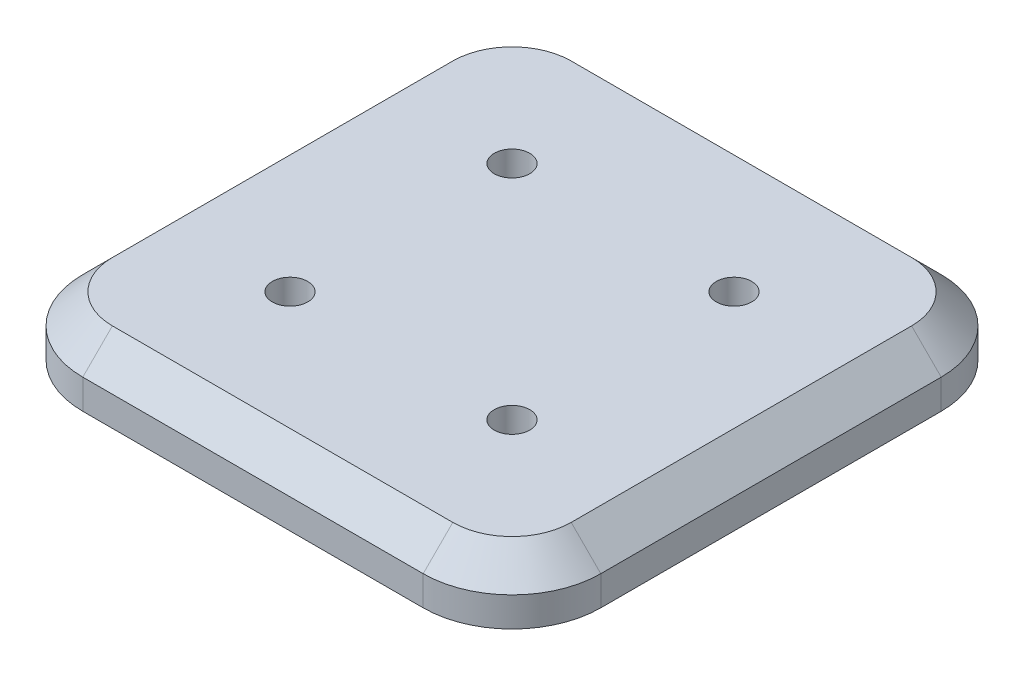
ISO-10303-21;
HEADER;
FILE_DESCRIPTION(('STEP AP214'),'2;1');
FILE_NAME('part.step','',(''),(''),'','','');
FILE_SCHEMA(('AUTOMOTIVE_DESIGN { 1 0 10303 214 1 1 1 1 }'));
ENDSEC;
DATA;
#1=APPLICATION_CONTEXT('core data for automotive mechanical design processes');
#2=APPLICATION_PROTOCOL_DEFINITION('international standard','automotive_design',2000,#1);
#3=PRODUCT_CONTEXT('',#1,'mechanical');
#4=PRODUCT('Part','Part','',(#3));
#5=PRODUCT_RELATED_PRODUCT_CATEGORY('part','',(#4));
#6=PRODUCT_DEFINITION_FORMATION('','',#4);
#7=PRODUCT_DEFINITION_CONTEXT('part definition',#1,'design');
#8=PRODUCT_DEFINITION('design','',#6,#7);
#9=PRODUCT_DEFINITION_SHAPE('','',#8);
#10=(LENGTH_UNIT() NAMED_UNIT(*) SI_UNIT(.MILLI.,.METRE.));
#11=(NAMED_UNIT(*) PLANE_ANGLE_UNIT() SI_UNIT($,.RADIAN.));
#12=(NAMED_UNIT(*) SI_UNIT($,.STERADIAN.) SOLID_ANGLE_UNIT());
#13=UNCERTAINTY_MEASURE_WITH_UNIT(LENGTH_MEASURE(1.E-05),#10,'distance_accuracy_value','');
#14=(GEOMETRIC_REPRESENTATION_CONTEXT(3) GLOBAL_UNCERTAINTY_ASSIGNED_CONTEXT((#13)) GLOBAL_UNIT_ASSIGNED_CONTEXT((#10,
#11,#12)) REPRESENTATION_CONTEXT('',''));
#15=CARTESIAN_POINT('',(0.,0.,0.));
#16=DIRECTION('',(0.,0.,1.));
#17=DIRECTION('',(1.,0.,0.));
#18=AXIS2_PLACEMENT_3D('',#15,#16,#17);
#19=CARTESIAN_POINT('',(87.5,20.,87.5));
#20=DIRECTION('',(-1.,0.,0.));
#21=DIRECTION('',(0.,0.,1.));
#22=AXIS2_PLACEMENT_3D('',#19,#20,#21);
#23=PLANE('',#22);
#24=DIRECTION('',(0.,-1.,0.));
#25=VECTOR('',#24,1.);
#26=CARTESIAN_POINT('',(87.5,20.,-57.5));
#27=LINE('',#26,#25);
#28=CARTESIAN_POINT('',(87.5,0.,-57.5));
#29=VERTEX_POINT('',#28);
#30=CARTESIAN_POINT('',(87.5,9.99999999999994,-57.5));
#31=VERTEX_POINT('',#30);
#32=EDGE_CURVE('E242',#29,#31,#27,.F.);
#33=ORIENTED_EDGE('',*,*,#32,.T.);
#34=DIRECTION('',(0.,0.,1.));
#35=VECTOR('',#34,1.);
#36=CARTESIAN_POINT('',(87.5,9.99999999999994,87.5));
#37=LINE('',#36,#35);
#38=CARTESIAN_POINT('',(87.5,9.99999999999994,57.5));
#39=VERTEX_POINT('',#38);
#40=EDGE_CURVE('E280',#31,#39,#37,.T.);
#41=ORIENTED_EDGE('',*,*,#40,.T.);
#42=DIRECTION('',(0.,-1.,0.));
#43=VECTOR('',#42,1.);
#44=CARTESIAN_POINT('',(87.5,20.,57.5));
#45=LINE('',#44,#43);
#46=CARTESIAN_POINT('',(87.5,0.,57.5));
#47=VERTEX_POINT('',#46);
#48=EDGE_CURVE('E245',#39,#47,#45,.T.);
#49=ORIENTED_EDGE('',*,*,#48,.T.);
#50=DIRECTION('',(0.,0.,-1.));
#51=VECTOR('',#50,1.);
#52=CARTESIAN_POINT('',(87.5,0.,87.5));
#53=LINE('',#52,#51);
#54=EDGE_CURVE('E215',#47,#29,#53,.T.);
#55=ORIENTED_EDGE('',*,*,#54,.T.);
#56=EDGE_LOOP('',(#33,#41,#49,#55));
#57=FACE_BOUND('',#56,.T.);
#58=ADVANCED_FACE('F41',(#57),#23,.F.);
#59=CARTESIAN_POINT('',(-87.5,20.,-87.5));
#60=DIRECTION('',(0.,0.,1.));
#61=DIRECTION('',(1.,0.,0.));
#62=AXIS2_PLACEMENT_3D('',#59,#60,#61);
#63=PLANE('',#62);
#64=DIRECTION('',(0.,-1.,0.));
#65=VECTOR('',#64,1.);
#66=CARTESIAN_POINT('',(-57.5,20.,-87.5));
#67=LINE('',#66,#65);
#68=CARTESIAN_POINT('',(-57.5,0.,-87.5));
#69=VERTEX_POINT('',#68);
#70=CARTESIAN_POINT('',(-57.5,9.99999999999994,-87.5));
#71=VERTEX_POINT('',#70);
#72=EDGE_CURVE('E237',#69,#71,#67,.F.);
#73=ORIENTED_EDGE('',*,*,#72,.T.);
#74=DIRECTION('',(1.,0.,0.));
#75=VECTOR('',#74,1.);
#76=CARTESIAN_POINT('',(-87.5,9.99999999999994,-87.5));
#77=LINE('',#76,#75);
#78=CARTESIAN_POINT('',(57.5,9.99999999999994,-87.5));
#79=VERTEX_POINT('',#78);
#80=EDGE_CURVE('E268',#71,#79,#77,.T.);
#81=ORIENTED_EDGE('',*,*,#80,.T.);
#82=DIRECTION('',(0.,-1.,0.));
#83=VECTOR('',#82,1.);
#84=CARTESIAN_POINT('',(57.5,20.,-87.5));
#85=LINE('',#84,#83);
#86=CARTESIAN_POINT('',(57.5,0.,-87.5));
#87=VERTEX_POINT('',#86);
#88=EDGE_CURVE('E240',#79,#87,#85,.T.);
#89=ORIENTED_EDGE('',*,*,#88,.T.);
#90=DIRECTION('',(-1.,0.,0.));
#91=VECTOR('',#90,1.);
#92=CARTESIAN_POINT('',(-87.5,0.,-87.5));
#93=LINE('',#92,#91);
#94=EDGE_CURVE('E213',#87,#69,#93,.T.);
#95=ORIENTED_EDGE('',*,*,#94,.T.);
#96=EDGE_LOOP('',(#73,#81,#89,#95));
#97=FACE_BOUND('',#96,.T.);
#98=ADVANCED_FACE('F346',(#97),#63,.F.);
#99=CARTESIAN_POINT('',(-87.5,20.,87.5));
#100=DIRECTION('',(1.,0.,0.));
#101=DIRECTION('',(0.,0.,-1.));
#102=AXIS2_PLACEMENT_3D('',#99,#100,#101);
#103=PLANE('',#102);
#104=DIRECTION('',(0.,-1.,0.));
#105=VECTOR('',#104,1.);
#106=CARTESIAN_POINT('',(-87.5,20.,57.5));
#107=LINE('',#106,#105);
#108=CARTESIAN_POINT('',(-87.5,0.,57.5));
#109=VERTEX_POINT('',#108);
#110=CARTESIAN_POINT('',(-87.5,9.99999999999994,57.5));
#111=VERTEX_POINT('',#110);
#112=EDGE_CURVE('E222',#109,#111,#107,.F.);
#113=ORIENTED_EDGE('',*,*,#112,.T.);
#114=DIRECTION('',(0.,0.,-1.));
#115=VECTOR('',#114,1.);
#116=CARTESIAN_POINT('',(-87.5,9.99999999999994,87.5));
#117=LINE('',#116,#115);
#118=CARTESIAN_POINT('',(-87.5,9.99999999999994,-57.5));
#119=VERTEX_POINT('',#118);
#120=EDGE_CURVE('E273',#111,#119,#117,.T.);
#121=ORIENTED_EDGE('',*,*,#120,.T.);
#122=DIRECTION('',(0.,-1.,0.));
#123=VECTOR('',#122,1.);
#124=CARTESIAN_POINT('',(-87.5,20.,-57.5));
#125=LINE('',#124,#123);
#126=CARTESIAN_POINT('',(-87.5,0.,-57.5));
#127=VERTEX_POINT('',#126);
#128=EDGE_CURVE('E227',#119,#127,#125,.T.);
#129=ORIENTED_EDGE('',*,*,#128,.T.);
#130=DIRECTION('',(0.,0.,1.));
#131=VECTOR('',#130,1.);
#132=CARTESIAN_POINT('',(-87.5,0.,87.5));
#133=LINE('',#132,#131);
#134=EDGE_CURVE('E218',#127,#109,#133,.T.);
#135=ORIENTED_EDGE('',*,*,#134,.T.);
#136=EDGE_LOOP('',(#113,#121,#129,#135));
#137=FACE_BOUND('',#136,.T.);
#138=ADVANCED_FACE('F319',(#137),#103,.F.);
#139=CARTESIAN_POINT('',(-87.5,20.,87.5));
#140=DIRECTION('',(0.,0.,-1.));
#141=DIRECTION('',(-1.,0.,0.));
#142=AXIS2_PLACEMENT_3D('',#139,#140,#141);
#143=PLANE('',#142);
#144=DIRECTION('',(0.,-1.,0.));
#145=VECTOR('',#144,1.);
#146=CARTESIAN_POINT('',(57.5,20.,87.5));
#147=LINE('',#146,#145);
#148=CARTESIAN_POINT('',(57.5,0.,87.5));
#149=VERTEX_POINT('',#148);
#150=CARTESIAN_POINT('',(57.5,9.99999999999994,87.5));
#151=VERTEX_POINT('',#150);
#152=EDGE_CURVE('E248',#149,#151,#147,.F.);
#153=ORIENTED_EDGE('',*,*,#152,.T.);
#154=DIRECTION('',(-1.,0.,0.));
#155=VECTOR('',#154,1.);
#156=CARTESIAN_POINT('',(-87.5,9.99999999999994,87.5));
#157=LINE('',#156,#155);
#158=CARTESIAN_POINT('',(-57.5,9.99999999999994,87.5));
#159=VERTEX_POINT('',#158);
#160=EDGE_CURVE('E11',#151,#159,#157,.T.);
#161=ORIENTED_EDGE('',*,*,#160,.T.);
#162=DIRECTION('',(0.,-1.,0.));
#163=VECTOR('',#162,1.);
#164=CARTESIAN_POINT('',(-57.5,20.,87.5));
#165=LINE('',#164,#163);
#166=CARTESIAN_POINT('',(-57.5,0.,87.5));
#167=VERTEX_POINT('',#166);
#168=EDGE_CURVE('E250',#159,#167,#165,.T.);
#169=ORIENTED_EDGE('',*,*,#168,.T.);
#170=DIRECTION('',(1.,0.,0.));
#171=VECTOR('',#170,1.);
#172=CARTESIAN_POINT('',(-87.5,0.,87.5));
#173=LINE('',#172,#171);
#174=EDGE_CURVE('E221',#167,#149,#173,.T.);
#175=ORIENTED_EDGE('',*,*,#174,.T.);
#176=EDGE_LOOP('',(#153,#161,#169,#175));
#177=FACE_BOUND('',#176,.T.);
#178=ADVANCED_FACE('F328',(#177),#143,.F.);
#179=CARTESIAN_POINT('',(0.,20.,0.));
#180=DIRECTION('',(0.,-1.,0.));
#181=DIRECTION('',(0.,0.,-1.));
#182=AXIS2_PLACEMENT_3D('',#179,#180,#181);
#183=PLANE('',#182);
#184=CARTESIAN_POINT('',(-37.5,20.,-37.5));
#185=DIRECTION('',(0.,1.,0.));
#186=DIRECTION('',(0.,0.,1.));
#187=AXIS2_PLACEMENT_3D('',#184,#185,#186);
#188=CIRCLE('',#187,5.99999999999998);
#189=CARTESIAN_POINT('',(-37.5,20.,-31.5));
#190=VERTEX_POINT('',#189);
#191=EDGE_CURVE('E190',#190,#190,#188,.T.);
#192=ORIENTED_EDGE('',*,*,#191,.F.);
#193=EDGE_LOOP('',(#192));
#194=FACE_BOUND('',#193,.T.);
#195=CARTESIAN_POINT('',(37.5,20.,-37.5));
#196=DIRECTION('',(0.,1.,0.));
#197=DIRECTION('',(0.,0.,1.));
#198=AXIS2_PLACEMENT_3D('',#195,#196,#197);
#199=CIRCLE('',#198,5.99999999999998);
#200=CARTESIAN_POINT('',(37.5,20.,-31.5));
#201=VERTEX_POINT('',#200);
#202=EDGE_CURVE('E194',#201,#201,#199,.T.);
#203=ORIENTED_EDGE('',*,*,#202,.F.);
#204=EDGE_LOOP('',(#203));
#205=FACE_BOUND('',#204,.T.);
#206=CARTESIAN_POINT('',(37.5,20.,37.5));
#207=DIRECTION('',(0.,1.,0.));
#208=DIRECTION('',(0.,0.,1.));
#209=AXIS2_PLACEMENT_3D('',#206,#207,#208);
#210=CIRCLE('',#209,5.99999999999998);
#211=CARTESIAN_POINT('',(37.5,20.,43.5));
#212=VERTEX_POINT('',#211);
#213=EDGE_CURVE('E197',#212,#212,#210,.T.);
#214=ORIENTED_EDGE('',*,*,#213,.F.);
#215=EDGE_LOOP('',(#214));
#216=FACE_BOUND('',#215,.T.);
#217=CARTESIAN_POINT('',(-37.5,20.,37.5));
#218=DIRECTION('',(0.,1.,0.));
#219=DIRECTION('',(0.,0.,1.));
#220=AXIS2_PLACEMENT_3D('',#217,#218,#219);
#221=CIRCLE('',#220,5.99999999999998);
#222=CARTESIAN_POINT('',(-37.5,20.,43.5));
#223=VERTEX_POINT('',#222);
#224=EDGE_CURVE('E204',#223,#223,#221,.T.);
#225=ORIENTED_EDGE('',*,*,#224,.F.);
#226=EDGE_LOOP('',(#225));
#227=FACE_BOUND('',#226,.T.);
#228=CARTESIAN_POINT('',(57.5,20.,-57.5));
#229=DIRECTION('',(0.,-1.,0.));
#230=DIRECTION('',(0.,0.,-1.));
#231=AXIS2_PLACEMENT_3D('',#228,#229,#230);
#232=CIRCLE('',#231,20.);
#233=CARTESIAN_POINT('',(77.5,20.,-57.5));
#234=VERTEX_POINT('',#233);
#235=CARTESIAN_POINT('',(57.5,20.,-77.5));
#236=VERTEX_POINT('',#235);
#237=EDGE_CURVE('E261',#234,#236,#232,.F.);
#238=ORIENTED_EDGE('',*,*,#237,.T.);
#239=DIRECTION('',(-1.,0.,0.));
#240=VECTOR('',#239,1.);
#241=CARTESIAN_POINT('',(0.,20.,-77.5));
#242=LINE('',#241,#240);
#243=CARTESIAN_POINT('',(-57.5,20.,-77.5));
#244=VERTEX_POINT('',#243);
#245=EDGE_CURVE('E264',#236,#244,#242,.T.);
#246=ORIENTED_EDGE('',*,*,#245,.T.);
#247=CARTESIAN_POINT('',(-57.5,20.,-57.5));
#248=DIRECTION('',(0.,-1.,0.));
#249=DIRECTION('',(0.,0.,-1.));
#250=AXIS2_PLACEMENT_3D('',#247,#248,#249);
#251=CIRCLE('',#250,20.);
#252=CARTESIAN_POINT('',(-77.5,20.,-57.5));
#253=VERTEX_POINT('',#252);
#254=EDGE_CURVE('E263',#244,#253,#251,.F.);
#255=ORIENTED_EDGE('',*,*,#254,.T.);
#256=DIRECTION('',(0.,0.,1.));
#257=VECTOR('',#256,1.);
#258=CARTESIAN_POINT('',(-77.5,20.,0.));
#259=LINE('',#258,#257);
#260=CARTESIAN_POINT('',(-77.5,20.,57.5));
#261=VERTEX_POINT('',#260);
#262=EDGE_CURVE('E256',#253,#261,#259,.T.);
#263=ORIENTED_EDGE('',*,*,#262,.T.);
#264=CARTESIAN_POINT('',(-57.5,20.,57.5));
#265=DIRECTION('',(0.,-1.,0.));
#266=DIRECTION('',(0.,0.,-1.));
#267=AXIS2_PLACEMENT_3D('',#264,#265,#266);
#268=CIRCLE('',#267,20.);
#269=CARTESIAN_POINT('',(-57.5,20.,77.5));
#270=VERTEX_POINT('',#269);
#271=EDGE_CURVE('E253',#261,#270,#268,.F.);
#272=ORIENTED_EDGE('',*,*,#271,.T.);
#273=DIRECTION('',(1.,0.,0.));
#274=VECTOR('',#273,1.);
#275=CARTESIAN_POINT('',(0.,20.,77.5));
#276=LINE('',#275,#274);
#277=CARTESIAN_POINT('',(57.5,20.,77.5));
#278=VERTEX_POINT('',#277);
#279=EDGE_CURVE('E252',#270,#278,#276,.T.);
#280=ORIENTED_EDGE('',*,*,#279,.T.);
#281=CARTESIAN_POINT('',(57.5,20.,57.5));
#282=DIRECTION('',(0.,-1.,0.));
#283=DIRECTION('',(0.,0.,-1.));
#284=AXIS2_PLACEMENT_3D('',#281,#282,#283);
#285=CIRCLE('',#284,20.);
#286=CARTESIAN_POINT('',(77.5,20.,57.5));
#287=VERTEX_POINT('',#286);
#288=EDGE_CURVE('E254',#278,#287,#285,.F.);
#289=ORIENTED_EDGE('',*,*,#288,.T.);
#290=DIRECTION('',(0.,0.,-1.));
#291=VECTOR('',#290,1.);
#292=CARTESIAN_POINT('',(77.5,20.,0.));
#293=LINE('',#292,#291);
#294=EDGE_CURVE('E260',#287,#234,#293,.T.);
#295=ORIENTED_EDGE('',*,*,#294,.T.);
#296=EDGE_LOOP('',(#238,#246,#255,#263,#272,#280,#289,#295));
#297=FACE_BOUND('',#296,.T.);
#298=ADVANCED_FACE('F356',(#194,#205,#216,#227,#297),#183,.F.);
#299=CARTESIAN_POINT('',(0.,0.,0.));
#300=DIRECTION('',(0.,-1.,0.));
#301=DIRECTION('',(0.,0.,-1.));
#302=AXIS2_PLACEMENT_3D('',#299,#300,#301);
#303=PLANE('',#302);
#304=CARTESIAN_POINT('',(-62.5,0.,62.5));
#305=DIRECTION('',(0.,-1.,0.));
#306=DIRECTION('',(0.,0.,-1.));
#307=AXIS2_PLACEMENT_3D('',#304,#305,#306);
#308=CIRCLE('',#307,5.99999999999998);
#309=CARTESIAN_POINT('',(-62.5,0.,56.5));
#310=VERTEX_POINT('',#309);
#311=EDGE_CURVE('E164',#310,#310,#308,.T.);
#312=ORIENTED_EDGE('',*,*,#311,.F.);
#313=EDGE_LOOP('',(#312));
#314=FACE_BOUND('',#313,.T.);
#315=CARTESIAN_POINT('',(62.5,0.,62.5));
#316=DIRECTION('',(0.,-1.,0.));
#317=DIRECTION('',(0.,0.,-1.));
#318=AXIS2_PLACEMENT_3D('',#315,#316,#317);
#319=CIRCLE('',#318,5.99999999999999);
#320=CARTESIAN_POINT('',(62.5,0.,56.5));
#321=VERTEX_POINT('',#320);
#322=EDGE_CURVE('E165',#321,#321,#319,.T.);
#323=ORIENTED_EDGE('',*,*,#322,.F.);
#324=EDGE_LOOP('',(#323));
#325=FACE_BOUND('',#324,.T.);
#326=CARTESIAN_POINT('',(62.5,0.,-62.5));
#327=DIRECTION('',(0.,-1.,0.));
#328=DIRECTION('',(0.,0.,-1.));
#329=AXIS2_PLACEMENT_3D('',#326,#327,#328);
#330=CIRCLE('',#329,5.99999999999999);
#331=CARTESIAN_POINT('',(62.5,0.,-68.5));
#332=VERTEX_POINT('',#331);
#333=EDGE_CURVE('E174',#332,#332,#330,.T.);
#334=ORIENTED_EDGE('',*,*,#333,.F.);
#335=EDGE_LOOP('',(#334));
#336=FACE_BOUND('',#335,.T.);
#337=CARTESIAN_POINT('',(-62.5,0.,-62.5));
#338=DIRECTION('',(0.,-1.,0.));
#339=DIRECTION('',(0.,0.,-1.));
#340=AXIS2_PLACEMENT_3D('',#337,#338,#339);
#341=CIRCLE('',#340,5.99999999999998);
#342=CARTESIAN_POINT('',(-62.5,0.,-68.5));
#343=VERTEX_POINT('',#342);
#344=EDGE_CURVE('E181',#343,#343,#341,.T.);
#345=ORIENTED_EDGE('',*,*,#344,.F.);
#346=EDGE_LOOP('',(#345));
#347=FACE_BOUND('',#346,.T.);
#348=ORIENTED_EDGE('',*,*,#134,.F.);
#349=CARTESIAN_POINT('',(-57.5,0.,-57.5));
#350=DIRECTION('',(0.,-1.,0.));
#351=DIRECTION('',(0.,0.,-1.));
#352=AXIS2_PLACEMENT_3D('',#349,#350,#351);
#353=CIRCLE('',#352,30.);
#354=EDGE_CURVE('E232',#127,#69,#353,.T.);
#355=ORIENTED_EDGE('',*,*,#354,.T.);
#356=ORIENTED_EDGE('',*,*,#94,.F.);
#357=CARTESIAN_POINT('',(57.5,0.,-57.5));
#358=DIRECTION('',(0.,-1.,0.));
#359=DIRECTION('',(0.,0.,-1.));
#360=AXIS2_PLACEMENT_3D('',#357,#358,#359);
#361=CIRCLE('',#360,30.);
#362=EDGE_CURVE('E231',#87,#29,#361,.T.);
#363=ORIENTED_EDGE('',*,*,#362,.T.);
#364=ORIENTED_EDGE('',*,*,#54,.F.);
#365=CARTESIAN_POINT('',(57.5,0.,57.5));
#366=DIRECTION('',(0.,-1.,0.));
#367=DIRECTION('',(0.,0.,-1.));
#368=AXIS2_PLACEMENT_3D('',#365,#366,#367);
#369=CIRCLE('',#368,30.);
#370=EDGE_CURVE('E233',#47,#149,#369,.T.);
#371=ORIENTED_EDGE('',*,*,#370,.T.);
#372=ORIENTED_EDGE('',*,*,#174,.F.);
#373=CARTESIAN_POINT('',(-57.5,0.,57.5));
#374=DIRECTION('',(0.,-1.,0.));
#375=DIRECTION('',(0.,0.,-1.));
#376=AXIS2_PLACEMENT_3D('',#373,#374,#375);
#377=CIRCLE('',#376,30.);
#378=EDGE_CURVE('E230',#167,#109,#377,.T.);
#379=ORIENTED_EDGE('',*,*,#378,.T.);
#380=EDGE_LOOP('',(#348,#355,#356,#363,#364,#371,#372,#379));
#381=FACE_BOUND('',#380,.T.);
#382=ADVANCED_FACE('F324',(#314,#325,#336,#347,#381),#303,.T.);
#383=CARTESIAN_POINT('',(-57.5,20.,-57.5));
#384=DIRECTION('',(0.,-1.,0.));
#385=DIRECTION('',(0.,0.,-1.));
#386=AXIS2_PLACEMENT_3D('',#383,#384,#385);
#387=CYLINDRICAL_SURFACE('',#386,30.);
#388=ORIENTED_EDGE('',*,*,#128,.F.);
#389=CARTESIAN_POINT('',(-57.5,9.99999999999994,-57.5));
#390=DIRECTION('',(0.,-1.,0.));
#391=DIRECTION('',(0.,0.,-1.));
#392=AXIS2_PLACEMENT_3D('',#389,#390,#391);
#393=CIRCLE('',#392,30.);
#394=EDGE_CURVE('E272',#119,#71,#393,.T.);
#395=ORIENTED_EDGE('',*,*,#394,.T.);
#396=ORIENTED_EDGE('',*,*,#72,.F.);
#397=ORIENTED_EDGE('',*,*,#354,.F.);
#398=EDGE_LOOP('',(#388,#395,#396,#397));
#399=FACE_BOUND('',#398,.T.);
#400=ADVANCED_FACE('F382',(#399),#387,.T.);
#401=CARTESIAN_POINT('',(57.5,20.,-57.5));
#402=DIRECTION('',(0.,-1.,0.));
#403=DIRECTION('',(0.,0.,-1.));
#404=AXIS2_PLACEMENT_3D('',#401,#402,#403);
#405=CYLINDRICAL_SURFACE('',#404,30.);
#406=ORIENTED_EDGE('',*,*,#88,.F.);
#407=CARTESIAN_POINT('',(57.5,9.99999999999994,-57.5));
#408=DIRECTION('',(0.,-1.,0.));
#409=DIRECTION('',(0.,0.,-1.));
#410=AXIS2_PLACEMENT_3D('',#407,#408,#409);
#411=CIRCLE('',#410,30.);
#412=EDGE_CURVE('E271',#79,#31,#411,.T.);
#413=ORIENTED_EDGE('',*,*,#412,.T.);
#414=ORIENTED_EDGE('',*,*,#32,.F.);
#415=ORIENTED_EDGE('',*,*,#362,.F.);
#416=EDGE_LOOP('',(#406,#413,#414,#415));
#417=FACE_BOUND('',#416,.T.);
#418=ADVANCED_FACE('F337',(#417),#405,.T.);
#419=CARTESIAN_POINT('',(57.5,20.,57.5));
#420=DIRECTION('',(0.,-1.,0.));
#421=DIRECTION('',(0.,0.,-1.));
#422=AXIS2_PLACEMENT_3D('',#419,#420,#421);
#423=CYLINDRICAL_SURFACE('',#422,30.);
#424=ORIENTED_EDGE('',*,*,#48,.F.);
#425=CARTESIAN_POINT('',(57.5,9.99999999999994,57.5));
#426=DIRECTION('',(0.,-1.,0.));
#427=DIRECTION('',(0.,0.,-1.));
#428=AXIS2_PLACEMENT_3D('',#425,#426,#427);
#429=CIRCLE('',#428,30.);
#430=EDGE_CURVE('E51',#39,#151,#429,.T.);
#431=ORIENTED_EDGE('',*,*,#430,.T.);
#432=ORIENTED_EDGE('',*,*,#152,.F.);
#433=ORIENTED_EDGE('',*,*,#370,.F.);
#434=EDGE_LOOP('',(#424,#431,#432,#433));
#435=FACE_BOUND('',#434,.T.);
#436=ADVANCED_FACE('F327',(#435),#423,.T.);
#437=CARTESIAN_POINT('',(-57.5,20.,57.5));
#438=DIRECTION('',(0.,-1.,0.));
#439=DIRECTION('',(0.,0.,-1.));
#440=AXIS2_PLACEMENT_3D('',#437,#438,#439);
#441=CYLINDRICAL_SURFACE('',#440,30.);
#442=ORIENTED_EDGE('',*,*,#168,.F.);
#443=CARTESIAN_POINT('',(-57.5,9.99999999999994,57.5));
#444=DIRECTION('',(0.,-1.,0.));
#445=DIRECTION('',(0.,0.,-1.));
#446=AXIS2_PLACEMENT_3D('',#443,#444,#445);
#447=CIRCLE('',#446,30.);
#448=EDGE_CURVE('E276',#159,#111,#447,.T.);
#449=ORIENTED_EDGE('',*,*,#448,.T.);
#450=ORIENTED_EDGE('',*,*,#112,.F.);
#451=ORIENTED_EDGE('',*,*,#378,.F.);
#452=EDGE_LOOP('',(#442,#449,#450,#451));
#453=FACE_BOUND('',#452,.T.);
#454=ADVANCED_FACE('F314',(#453),#441,.T.);
#455=CARTESIAN_POINT('',(0.,20.,77.5));
#456=DIRECTION('',(0.,-0.707106781186545,-0.707106781186551));
#457=DIRECTION('',(1.,0.,0.));
#458=AXIS2_PLACEMENT_3D('',#455,#456,#457);
#459=PLANE('',#458);
#460=DIRECTION('',(0.,0.707106781186551,-0.707106781186545));
#461=VECTOR('',#460,1.);
#462=CARTESIAN_POINT('',(-57.5,9.99999999999994,87.5));
#463=LINE('',#462,#461);
#464=EDGE_CURVE('E298',#159,#270,#463,.T.);
#465=ORIENTED_EDGE('',*,*,#464,.F.);
#466=ORIENTED_EDGE('',*,*,#160,.F.);
#467=DIRECTION('',(0.,-0.707106781186551,0.707106781186545));
#468=VECTOR('',#467,1.);
#469=CARTESIAN_POINT('',(57.5,20.,77.5));
#470=LINE('',#469,#468);
#471=EDGE_CURVE('E46',#278,#151,#470,.T.);
#472=ORIENTED_EDGE('',*,*,#471,.F.);
#473=ORIENTED_EDGE('',*,*,#279,.F.);
#474=EDGE_LOOP('',(#465,#466,#472,#473));
#475=FACE_BOUND('',#474,.T.);
#476=ADVANCED_FACE('F42',(#475),#459,.F.);
#477=CARTESIAN_POINT('',(57.5,20.,57.5));
#478=DIRECTION('',(0.,-1.,0.));
#479=DIRECTION('',(0.,0.,-1.));
#480=AXIS2_PLACEMENT_3D('',#477,#478,#479);
#481=CONICAL_SURFACE('',#480,20.,0.785398163397444);
#482=ORIENTED_EDGE('',*,*,#471,.T.);
#483=ORIENTED_EDGE('',*,*,#430,.F.);
#484=DIRECTION('',(0.707106781186545,-0.707106781186551,0.));
#485=VECTOR('',#484,1.);
#486=CARTESIAN_POINT('',(77.5,20.,57.5));
#487=LINE('',#486,#485);
#488=EDGE_CURVE('E295',#287,#39,#487,.T.);
#489=ORIENTED_EDGE('',*,*,#488,.F.);
#490=ORIENTED_EDGE('',*,*,#288,.F.);
#491=EDGE_LOOP('',(#482,#483,#489,#490));
#492=FACE_BOUND('',#491,.T.);
#493=ADVANCED_FACE('F306',(#492),#481,.T.);
#494=CARTESIAN_POINT('',(-57.5,20.,57.5));
#495=DIRECTION('',(0.,-1.,0.));
#496=DIRECTION('',(0.,0.,-1.));
#497=AXIS2_PLACEMENT_3D('',#494,#495,#496);
#498=CONICAL_SURFACE('',#497,20.,0.785398163397444);
#499=ORIENTED_EDGE('',*,*,#464,.T.);
#500=ORIENTED_EDGE('',*,*,#271,.F.);
#501=DIRECTION('',(0.707106781186545,0.707106781186551,0.));
#502=VECTOR('',#501,1.);
#503=CARTESIAN_POINT('',(-87.5,9.99999999999994,57.5));
#504=LINE('',#503,#502);
#505=EDGE_CURVE('E293',#111,#261,#504,.T.);
#506=ORIENTED_EDGE('',*,*,#505,.F.);
#507=ORIENTED_EDGE('',*,*,#448,.F.);
#508=EDGE_LOOP('',(#499,#500,#506,#507));
#509=FACE_BOUND('',#508,.T.);
#510=ADVANCED_FACE('F311',(#509),#498,.T.);
#511=CARTESIAN_POINT('',(77.5,20.,0.));
#512=DIRECTION('',(-0.707106781186551,-0.707106781186545,0.));
#513=DIRECTION('',(0.,0.,-1.));
#514=AXIS2_PLACEMENT_3D('',#511,#512,#513);
#515=PLANE('',#514);
#516=ORIENTED_EDGE('',*,*,#488,.T.);
#517=ORIENTED_EDGE('',*,*,#40,.F.);
#518=DIRECTION('',(0.707106781186545,-0.707106781186551,0.));
#519=VECTOR('',#518,1.);
#520=CARTESIAN_POINT('',(77.5,20.,-57.5));
#521=LINE('',#520,#519);
#522=EDGE_CURVE('E288',#234,#31,#521,.T.);
#523=ORIENTED_EDGE('',*,*,#522,.F.);
#524=ORIENTED_EDGE('',*,*,#294,.F.);
#525=EDGE_LOOP('',(#516,#517,#523,#524));
#526=FACE_BOUND('',#525,.T.);
#527=ADVANCED_FACE('F363',(#526),#515,.F.);
#528=CARTESIAN_POINT('',(-77.5,20.,0.));
#529=DIRECTION('',(0.707106781186551,-0.707106781186545,0.));
#530=DIRECTION('',(0.,0.,1.));
#531=AXIS2_PLACEMENT_3D('',#528,#529,#530);
#532=PLANE('',#531);
#533=ORIENTED_EDGE('',*,*,#505,.T.);
#534=ORIENTED_EDGE('',*,*,#262,.F.);
#535=DIRECTION('',(0.707106781186545,0.707106781186551,0.));
#536=VECTOR('',#535,1.);
#537=CARTESIAN_POINT('',(-87.5,9.99999999999994,-57.5));
#538=LINE('',#537,#536);
#539=EDGE_CURVE('E284',#119,#253,#538,.T.);
#540=ORIENTED_EDGE('',*,*,#539,.F.);
#541=ORIENTED_EDGE('',*,*,#120,.F.);
#542=EDGE_LOOP('',(#533,#534,#540,#541));
#543=FACE_BOUND('',#542,.T.);
#544=ADVANCED_FACE('F361',(#543),#532,.F.);
#545=CARTESIAN_POINT('',(57.5,20.,-57.5));
#546=DIRECTION('',(0.,-1.,0.));
#547=DIRECTION('',(0.,0.,-1.));
#548=AXIS2_PLACEMENT_3D('',#545,#546,#547);
#549=CONICAL_SURFACE('',#548,20.,0.785398163397444);
#550=ORIENTED_EDGE('',*,*,#522,.T.);
#551=ORIENTED_EDGE('',*,*,#412,.F.);
#552=DIRECTION('',(0.,-0.707106781186551,-0.707106781186545));
#553=VECTOR('',#552,1.);
#554=CARTESIAN_POINT('',(57.5,20.,-77.5));
#555=LINE('',#554,#553);
#556=EDGE_CURVE('E283',#236,#79,#555,.T.);
#557=ORIENTED_EDGE('',*,*,#556,.F.);
#558=ORIENTED_EDGE('',*,*,#237,.F.);
#559=EDGE_LOOP('',(#550,#551,#557,#558));
#560=FACE_BOUND('',#559,.T.);
#561=ADVANCED_FACE('F338',(#560),#549,.T.);
#562=CARTESIAN_POINT('',(-57.5,20.,-57.5));
#563=DIRECTION('',(0.,-1.,0.));
#564=DIRECTION('',(0.,0.,-1.));
#565=AXIS2_PLACEMENT_3D('',#562,#563,#564);
#566=CONICAL_SURFACE('',#565,20.,0.785398163397444);
#567=ORIENTED_EDGE('',*,*,#539,.T.);
#568=ORIENTED_EDGE('',*,*,#254,.F.);
#569=DIRECTION('',(0.,0.707106781186551,0.707106781186545));
#570=VECTOR('',#569,1.);
#571=CARTESIAN_POINT('',(-57.5,9.99999999999994,-87.5));
#572=LINE('',#571,#570);
#573=EDGE_CURVE('E212',#71,#244,#572,.T.);
#574=ORIENTED_EDGE('',*,*,#573,.F.);
#575=ORIENTED_EDGE('',*,*,#394,.F.);
#576=EDGE_LOOP('',(#567,#568,#574,#575));
#577=FACE_BOUND('',#576,.T.);
#578=ADVANCED_FACE('F352',(#577),#566,.T.);
#579=CARTESIAN_POINT('',(0.,20.,-77.5));
#580=DIRECTION('',(0.,-0.707106781186545,0.707106781186551));
#581=DIRECTION('',(-1.,0.,0.));
#582=AXIS2_PLACEMENT_3D('',#579,#580,#581);
#583=PLANE('',#582);
#584=ORIENTED_EDGE('',*,*,#556,.T.);
#585=ORIENTED_EDGE('',*,*,#80,.F.);
#586=ORIENTED_EDGE('',*,*,#573,.T.);
#587=ORIENTED_EDGE('',*,*,#245,.F.);
#588=EDGE_LOOP('',(#584,#585,#586,#587));
#589=FACE_BOUND('',#588,.T.);
#590=ADVANCED_FACE('F349',(#589),#583,.F.);
#591=CARTESIAN_POINT('',(-37.5,10.,37.5));
#592=DIRECTION('',(0.,1.,0.));
#593=DIRECTION('',(0.,0.,1.));
#594=AXIS2_PLACEMENT_3D('',#591,#592,#593);
#595=CONICAL_SURFACE('',#594,5.99999999999998,1.02974425867665);
#596=CARTESIAN_POINT('',(-37.5,6.39483628583465,37.5));
#597=VERTEX_POINT('',#596);
#598=VERTEX_LOOP('',#597);
#599=FACE_BOUND('',#598,.T.);
#600=CARTESIAN_POINT('',(-37.5,10.,37.5));
#601=DIRECTION('',(0.,1.,0.));
#602=DIRECTION('',(0.,0.,1.));
#603=AXIS2_PLACEMENT_3D('',#600,#601,#602);
#604=CIRCLE('',#603,5.99999999999998);
#605=CARTESIAN_POINT('',(-37.5,10.,43.5));
#606=VERTEX_POINT('',#605);
#607=EDGE_CURVE('E206',#606,#606,#604,.T.);
#608=ORIENTED_EDGE('',*,*,#607,.T.);
#609=EDGE_LOOP('',(#608));
#610=FACE_BOUND('',#609,.T.);
#611=ADVANCED_FACE('F400',(#599,#610),#595,.F.);
#612=CARTESIAN_POINT('',(-37.5,20.,37.5));
#613=DIRECTION('',(0.,1.,0.));
#614=DIRECTION('',(0.,0.,1.));
#615=AXIS2_PLACEMENT_3D('',#612,#613,#614);
#616=CYLINDRICAL_SURFACE('',#615,5.99999999999998);
#617=ORIENTED_EDGE('',*,*,#607,.F.);
#618=EDGE_LOOP('',(#617));
#619=FACE_BOUND('',#618,.T.);
#620=ORIENTED_EDGE('',*,*,#224,.T.);
#621=EDGE_LOOP('',(#620));
#622=FACE_BOUND('',#621,.T.);
#623=ADVANCED_FACE('F535',(#619,#622),#616,.F.);
#624=CARTESIAN_POINT('',(37.5,10.,37.5));
#625=DIRECTION('',(0.,1.,0.));
#626=DIRECTION('',(0.,0.,1.));
#627=AXIS2_PLACEMENT_3D('',#624,#625,#626);
#628=CONICAL_SURFACE('',#627,5.99999999999998,1.02974425867665);
#629=CARTESIAN_POINT('',(37.5,6.39483628583465,37.5));
#630=VERTEX_POINT('',#629);
#631=VERTEX_LOOP('',#630);
#632=FACE_BOUND('',#631,.T.);
#633=CARTESIAN_POINT('',(37.5,10.,37.5));
#634=DIRECTION('',(0.,1.,0.));
#635=DIRECTION('',(0.,0.,1.));
#636=AXIS2_PLACEMENT_3D('',#633,#634,#635);
#637=CIRCLE('',#636,5.99999999999998);
#638=CARTESIAN_POINT('',(37.5,10.,43.5));
#639=VERTEX_POINT('',#638);
#640=EDGE_CURVE('E205',#639,#639,#637,.T.);
#641=ORIENTED_EDGE('',*,*,#640,.T.);
#642=EDGE_LOOP('',(#641));
#643=FACE_BOUND('',#642,.T.);
#644=ADVANCED_FACE('F541',(#632,#643),#628,.F.);
#645=CARTESIAN_POINT('',(37.5,20.,37.5));
#646=DIRECTION('',(0.,1.,0.));
#647=DIRECTION('',(0.,0.,1.));
#648=AXIS2_PLACEMENT_3D('',#645,#646,#647);
#649=CYLINDRICAL_SURFACE('',#648,5.99999999999998);
#650=ORIENTED_EDGE('',*,*,#640,.F.);
#651=EDGE_LOOP('',(#650));
#652=FACE_BOUND('',#651,.T.);
#653=ORIENTED_EDGE('',*,*,#213,.T.);
#654=EDGE_LOOP('',(#653));
#655=FACE_BOUND('',#654,.T.);
#656=ADVANCED_FACE('F549',(#652,#655),#649,.F.);
#657=CARTESIAN_POINT('',(37.5,10.,-37.5));
#658=DIRECTION('',(0.,1.,0.));
#659=DIRECTION('',(0.,0.,1.));
#660=AXIS2_PLACEMENT_3D('',#657,#658,#659);
#661=CONICAL_SURFACE('',#660,5.99999999999998,1.02974425867665);
#662=CARTESIAN_POINT('',(37.5,6.39483628583465,-37.5));
#663=VERTEX_POINT('',#662);
#664=VERTEX_LOOP('',#663);
#665=FACE_BOUND('',#664,.T.);
#666=CARTESIAN_POINT('',(37.5,10.,-37.5));
#667=DIRECTION('',(0.,1.,0.));
#668=DIRECTION('',(0.,0.,1.));
#669=AXIS2_PLACEMENT_3D('',#666,#667,#668);
#670=CIRCLE('',#669,5.99999999999998);
#671=CARTESIAN_POINT('',(37.5,10.,-31.5));
#672=VERTEX_POINT('',#671);
#673=EDGE_CURVE('E196',#672,#672,#670,.T.);
#674=ORIENTED_EDGE('',*,*,#673,.T.);
#675=EDGE_LOOP('',(#674));
#676=FACE_BOUND('',#675,.T.);
#677=ADVANCED_FACE('F559',(#665,#676),#661,.F.);
#678=CARTESIAN_POINT('',(37.5,20.,-37.5));
#679=DIRECTION('',(0.,1.,0.));
#680=DIRECTION('',(0.,0.,1.));
#681=AXIS2_PLACEMENT_3D('',#678,#679,#680);
#682=CYLINDRICAL_SURFACE('',#681,5.99999999999998);
#683=ORIENTED_EDGE('',*,*,#673,.F.);
#684=EDGE_LOOP('',(#683));
#685=FACE_BOUND('',#684,.T.);
#686=ORIENTED_EDGE('',*,*,#202,.T.);
#687=EDGE_LOOP('',(#686));
#688=FACE_BOUND('',#687,.T.);
#689=ADVANCED_FACE('F568',(#685,#688),#682,.F.);
#690=CARTESIAN_POINT('',(-37.5,10.,-37.5));
#691=DIRECTION('',(0.,1.,0.));
#692=DIRECTION('',(0.,0.,1.));
#693=AXIS2_PLACEMENT_3D('',#690,#691,#692);
#694=CONICAL_SURFACE('',#693,5.99999999999998,1.02974425867665);
#695=CARTESIAN_POINT('',(-37.5,6.39483628583465,-37.5));
#696=VERTEX_POINT('',#695);
#697=VERTEX_LOOP('',#696);
#698=FACE_BOUND('',#697,.T.);
#699=CARTESIAN_POINT('',(-37.5,10.,-37.5));
#700=DIRECTION('',(0.,1.,0.));
#701=DIRECTION('',(0.,0.,1.));
#702=AXIS2_PLACEMENT_3D('',#699,#700,#701);
#703=CIRCLE('',#702,5.99999999999998);
#704=CARTESIAN_POINT('',(-37.5,10.,-31.5));
#705=VERTEX_POINT('',#704);
#706=EDGE_CURVE('E188',#705,#705,#703,.T.);
#707=ORIENTED_EDGE('',*,*,#706,.T.);
#708=EDGE_LOOP('',(#707));
#709=FACE_BOUND('',#708,.T.);
#710=ADVANCED_FACE('F580',(#698,#709),#694,.F.);
#711=CARTESIAN_POINT('',(-37.5,20.,-37.5));
#712=DIRECTION('',(0.,1.,0.));
#713=DIRECTION('',(0.,0.,1.));
#714=AXIS2_PLACEMENT_3D('',#711,#712,#713);
#715=CYLINDRICAL_SURFACE('',#714,5.99999999999998);
#716=ORIENTED_EDGE('',*,*,#706,.F.);
#717=EDGE_LOOP('',(#716));
#718=FACE_BOUND('',#717,.T.);
#719=ORIENTED_EDGE('',*,*,#191,.T.);
#720=EDGE_LOOP('',(#719));
#721=FACE_BOUND('',#720,.T.);
#722=ADVANCED_FACE('F586',(#718,#721),#715,.F.);
#723=CARTESIAN_POINT('',(-62.5,9.99999999999999,-62.5));
#724=DIRECTION('',(0.,-1.,0.));
#725=DIRECTION('',(0.,0.,-1.));
#726=AXIS2_PLACEMENT_3D('',#723,#724,#725);
#727=CONICAL_SURFACE('',#726,5.99999999999998,1.02974425867665);
#728=CARTESIAN_POINT('',(-62.5,13.6051637141654,-62.5));
#729=VERTEX_POINT('',#728);
#730=VERTEX_LOOP('',#729);
#731=FACE_BOUND('',#730,.T.);
#732=CARTESIAN_POINT('',(-62.5,9.99999999999999,-62.5));
#733=DIRECTION('',(0.,-1.,0.));
#734=DIRECTION('',(0.,0.,-1.));
#735=AXIS2_PLACEMENT_3D('',#732,#733,#734);
#736=CIRCLE('',#735,5.99999999999998);
#737=CARTESIAN_POINT('',(-62.5,9.99999999999999,-68.5));
#738=VERTEX_POINT('',#737);
#739=EDGE_CURVE('E183',#738,#738,#736,.T.);
#740=ORIENTED_EDGE('',*,*,#739,.T.);
#741=EDGE_LOOP('',(#740));
#742=FACE_BOUND('',#741,.T.);
#743=ADVANCED_FACE('F594',(#731,#742),#727,.F.);
#744=CARTESIAN_POINT('',(-62.5,0.,-62.5));
#745=DIRECTION('',(0.,-1.,0.));
#746=DIRECTION('',(0.,0.,-1.));
#747=AXIS2_PLACEMENT_3D('',#744,#745,#746);
#748=CYLINDRICAL_SURFACE('',#747,5.99999999999998);
#749=ORIENTED_EDGE('',*,*,#739,.F.);
#750=EDGE_LOOP('',(#749));
#751=FACE_BOUND('',#750,.T.);
#752=ORIENTED_EDGE('',*,*,#344,.T.);
#753=EDGE_LOOP('',(#752));
#754=FACE_BOUND('',#753,.T.);
#755=ADVANCED_FACE('F601',(#751,#754),#748,.F.);
#756=CARTESIAN_POINT('',(62.5,9.99999999999999,-62.5));
#757=DIRECTION('',(0.,-1.,0.));
#758=DIRECTION('',(0.,0.,-1.));
#759=AXIS2_PLACEMENT_3D('',#756,#757,#758);
#760=CONICAL_SURFACE('',#759,5.99999999999999,1.02974425867665);
#761=CARTESIAN_POINT('',(62.5,13.6051637141654,-62.5));
#762=VERTEX_POINT('',#761);
#763=VERTEX_LOOP('',#762);
#764=FACE_BOUND('',#763,.T.);
#765=CARTESIAN_POINT('',(62.5,9.99999999999999,-62.5));
#766=DIRECTION('',(0.,-1.,0.));
#767=DIRECTION('',(0.,0.,-1.));
#768=AXIS2_PLACEMENT_3D('',#765,#766,#767);
#769=CIRCLE('',#768,5.99999999999999);
#770=CARTESIAN_POINT('',(62.5,9.99999999999999,-68.5));
#771=VERTEX_POINT('',#770);
#772=EDGE_CURVE('E178',#771,#771,#769,.T.);
#773=ORIENTED_EDGE('',*,*,#772,.T.);
#774=EDGE_LOOP('',(#773));
#775=FACE_BOUND('',#774,.T.);
#776=ADVANCED_FACE('F613',(#764,#775),#760,.F.);
#777=CARTESIAN_POINT('',(62.5,0.,-62.5));
#778=DIRECTION('',(0.,-1.,0.));
#779=DIRECTION('',(0.,0.,-1.));
#780=AXIS2_PLACEMENT_3D('',#777,#778,#779);
#781=CYLINDRICAL_SURFACE('',#780,5.99999999999999);
#782=ORIENTED_EDGE('',*,*,#772,.F.);
#783=EDGE_LOOP('',(#782));
#784=FACE_BOUND('',#783,.T.);
#785=ORIENTED_EDGE('',*,*,#333,.T.);
#786=EDGE_LOOP('',(#785));
#787=FACE_BOUND('',#786,.T.);
#788=ADVANCED_FACE('F625',(#784,#787),#781,.F.);
#789=CARTESIAN_POINT('',(62.5,9.99999999999999,62.5));
#790=DIRECTION('',(0.,-1.,0.));
#791=DIRECTION('',(0.,0.,-1.));
#792=AXIS2_PLACEMENT_3D('',#789,#790,#791);
#793=CONICAL_SURFACE('',#792,5.99999999999999,1.02974425867665);
#794=CARTESIAN_POINT('',(62.5,13.6051637141654,62.5));
#795=VERTEX_POINT('',#794);
#796=VERTEX_LOOP('',#795);
#797=FACE_BOUND('',#796,.T.);
#798=CARTESIAN_POINT('',(62.5,9.99999999999999,62.5));
#799=DIRECTION('',(0.,-1.,0.));
#800=DIRECTION('',(0.,0.,-1.));
#801=AXIS2_PLACEMENT_3D('',#798,#799,#800);
#802=CIRCLE('',#801,5.99999999999999);
#803=CARTESIAN_POINT('',(62.5,9.99999999999999,56.5));
#804=VERTEX_POINT('',#803);
#805=EDGE_CURVE('E166',#804,#804,#802,.T.);
#806=ORIENTED_EDGE('',*,*,#805,.T.);
#807=EDGE_LOOP('',(#806));
#808=FACE_BOUND('',#807,.T.);
#809=ADVANCED_FACE('F631',(#797,#808),#793,.F.);
#810=CARTESIAN_POINT('',(62.5,0.,62.5));
#811=DIRECTION('',(0.,-1.,0.));
#812=DIRECTION('',(0.,0.,-1.));
#813=AXIS2_PLACEMENT_3D('',#810,#811,#812);
#814=CYLINDRICAL_SURFACE('',#813,5.99999999999999);
#815=ORIENTED_EDGE('',*,*,#805,.F.);
#816=EDGE_LOOP('',(#815));
#817=FACE_BOUND('',#816,.T.);
#818=ORIENTED_EDGE('',*,*,#322,.T.);
#819=EDGE_LOOP('',(#818));
#820=FACE_BOUND('',#819,.T.);
#821=ADVANCED_FACE('F158',(#817,#820),#814,.F.);
#822=CARTESIAN_POINT('',(-62.5,9.99999999999999,62.5));
#823=DIRECTION('',(0.,-1.,0.));
#824=DIRECTION('',(0.,0.,-1.));
#825=AXIS2_PLACEMENT_3D('',#822,#823,#824);
#826=CONICAL_SURFACE('',#825,5.99999999999998,1.02974425867665);
#827=CARTESIAN_POINT('',(-62.5,13.6051637141654,62.5));
#828=VERTEX_POINT('',#827);
#829=VERTEX_LOOP('',#828);
#830=FACE_BOUND('',#829,.T.);
#831=CARTESIAN_POINT('',(-62.5,9.99999999999999,62.5));
#832=DIRECTION('',(0.,-1.,0.));
#833=DIRECTION('',(0.,0.,-1.));
#834=AXIS2_PLACEMENT_3D('',#831,#832,#833);
#835=CIRCLE('',#834,5.99999999999998);
#836=CARTESIAN_POINT('',(-62.5,9.99999999999999,56.5));
#837=VERTEX_POINT('',#836);
#838=EDGE_CURVE('E162',#837,#837,#835,.T.);
#839=ORIENTED_EDGE('',*,*,#838,.T.);
#840=EDGE_LOOP('',(#839));
#841=FACE_BOUND('',#840,.T.);
#842=ADVANCED_FACE('F152',(#830,#841),#826,.F.);
#843=CARTESIAN_POINT('',(-62.5,0.,62.5));
#844=DIRECTION('',(0.,-1.,0.));
#845=DIRECTION('',(0.,0.,-1.));
#846=AXIS2_PLACEMENT_3D('',#843,#844,#845);
#847=CYLINDRICAL_SURFACE('',#846,5.99999999999998);
#848=ORIENTED_EDGE('',*,*,#838,.F.);
#849=EDGE_LOOP('',(#848));
#850=FACE_BOUND('',#849,.T.);
#851=ORIENTED_EDGE('',*,*,#311,.T.);
#852=EDGE_LOOP('',(#851));
#853=FACE_BOUND('',#852,.T.);
#854=ADVANCED_FACE('F160',(#850,#853),#847,.F.);
#855=CLOSED_SHELL('',(#58,#98,#138,#178,#298,#382,#400,#418,#436,#454,#476,#493,#510,#527,#544,
#561,#578,#590,#611,#623,#644,#656,#677,#689,#710,#722,#743,#755,#776,#788,#809,#821,#842,#854));
#856=MANIFOLD_SOLID_BREP('B2',#855);
#857=ADVANCED_BREP_SHAPE_REPRESENTATION('',(#18,#856),#14);
#858=SHAPE_DEFINITION_REPRESENTATION(#9,#857);
ENDSEC;
END-ISO-10303-21;
